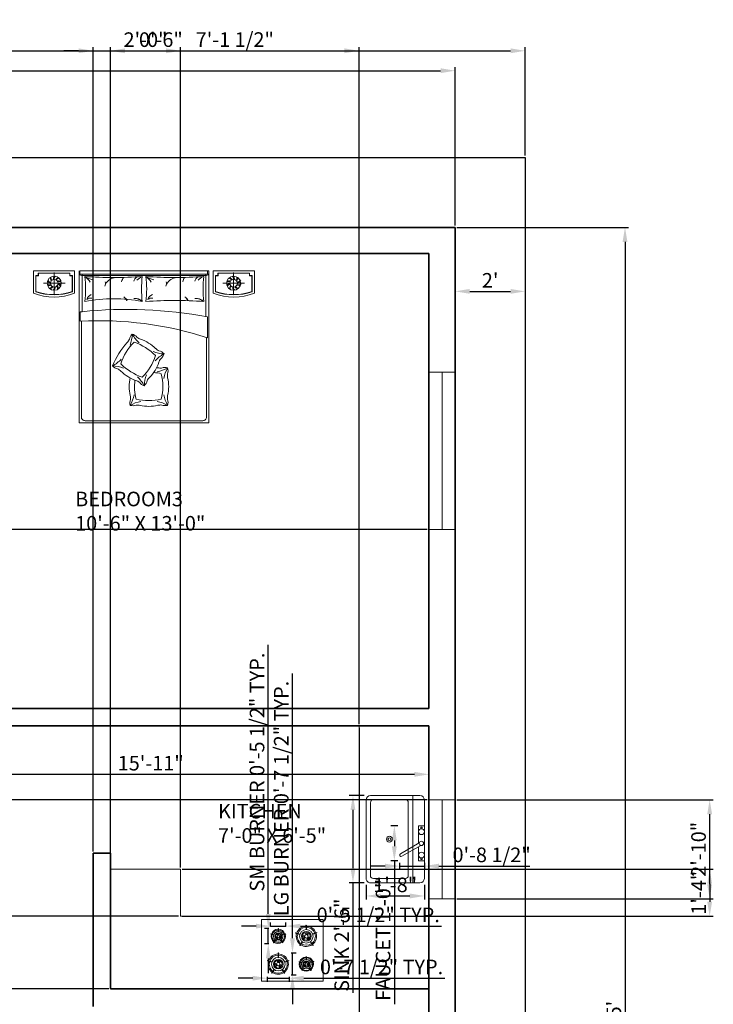
# Model space of a CAD drawing. Units: inches. Extents: x -938 to -211, y -366 to 366.
# Tile 4 of 4: x -450 to -211, y 4 to 341. Entities that reach past the tile are written whole.
import ezdxf

# ---------------------------------------------------------------- set-up
doc = ezdxf.new("R2010")
doc.units = ezdxf.units.IN
doc.header["$PDMODE"] = 35
doc.header["$PDSIZE"] = 5
for name, color, linetype, lineweight in [('A-ANNO-DIMS', 2, 'Continuous', 18), ('A-AREA-IDEN', 7, 'Continuous', 18), ('A-EQPM', 8, 'Continuous', 18), ('A-FLOR-CASE', 32, 'Continuous', 18), ('A-FLOR-FIXT', 9, 'Continuous', 18), ('A-GLAZ', 4, 'Continuous', 18), ('A-WALL', 7, 'Continuous', 35), ('C-PROP', 8, 'Continuous', 25), ('furn', 28, 'Continuous', 13)]:
    doc.layers.add(name, color=color, linetype=linetype, lineweight=lineweight)
doc.styles.get("Standard").update_dxf_attribs({"font": 'arial.ttf'})
doc.dimstyles.new('ISO-25', dxfattribs={"dimtxt": 5, "dimasz": 5, "dimexe": 1.25, "dimexo": 0.625, "dimtad": 1, "dimlunit": 3, "dimtxsty": 'Standard', "dimcen": 2.5, "dimadec": 0, "dimazin": 0, "dimtfac": 1, "dimtmove": 0, "dimatfit": 3, "dimfxl": 1, "dimarcsym": 0})

# ---------------------------------------------------------------- blocks, each defined once
blk = doc.blocks.new('Sink-single - 30 in top')
blk.add_line((-15, -3.999996), (15, -3.999996))
for points in [[(-13.5, 0), (13.5, 0)], [(-15, -18.499996), (-15, -1.5)], [(15, -1.5), (15, -18.499996)], [(-13.5, -17.499996), (-13.5, -6.499996)], [(-12.5, -5.499996), (12.5, -5.499996)], [(13.5, -6.499996), (13.5, -17.499996)], [(13.5, -19.999996), (-13.5, -19.999996)], [(12.5, -18.499996), (-12.5, -18.499996)]]:
    blk.add_lwpolyline(points)
for radius in [1, 0.5]:
    blk.add_circle((0, -11.999996), radius)
for centre, radius, start, end in [((-13.5, -1.5), 1.5, 90, 180), ((13.5, -1.5), 1.5, 0, 90), ((-12.5, -6.499996), 1, 90, 180), ((12.5, -6.499996), 1, 0, 90), ((-13.5, -18.499996), 1.5, 180, 270), ((-12.5, -17.499996), 1, 180, 270), ((12.5, -17.499996), 1, 270, 0), ((13.5, -18.499996), 1.5, 270, 0)]:
    blk.add_arc(centre, radius, start, end)
blk = doc.blocks.new('Faucet - kit sink top')
for p, q in [((-5.5, -0.75), (-5.5, -1.25)), ((-4.94278, -0.75), (-5.5, -0.75)), ((-5.5, -1.25), (-4.94278, -1.25)), ((-0.14775, -1.7441), (3.56698, -8.1782)), ((4.43301, -7.6782), (0.71828, -1.2441)), ((4.94278, -0.75), (5.5, -0.75)), ((5.5, -1.25), (4.94278, -1.25)), ((5.5, -0.75), (5.5, -1.25))]:
    blk.add_line(p, q)
blk.add_lwpolyline([(-0.00587, -2), (-6, -2), (-6, 0), (6, 0), (6, -2), (1.15195, -2)])
for centre, radius in [((-4, -1), 1), ((4, -1), 1), ((0, -1), 0.75)]:
    blk.add_circle(centre, radius)
blk.add_arc((4, -7.9282), 0.5, 210, 30)
blk = doc.blocks.new('*D9')
at = {"layer": 'A-ANNO-DIMS', "color": 0, "lineweight": -2, "transparency": 16777216}
for p, q in [((-500.06, 98.36), (-500.06, 81.14)), ((-309.06, 98.36), (-309.06, 81.14)), ((-495.06, 82.39), (-314.06, 82.39))]:
    blk.add_line(p, q, dxfattribs=at)
at = {"layer": 'A-ANNO-DIMS', "color": 0, "transparency": 16777216}
for points in [[(-495.06, 83.22), (-495.06, 81.55), (-500.06, 82.39)], [(-314.06, 83.22), (-314.06, 81.55), (-309.06, 82.39)]]:
    blk.add_solid(points, dxfattribs=at)
at = {"layer": 'Defpoints', "color": 0, "transparency": 16777216}
for p in [(-500.06, 98.98), (-309.06, 98.98), (-309.06, 82.39)]:
    blk.add_point(p, dxfattribs=at)
at = {"layer": 'A-ANNO-DIMS', "color": 0, "transparency": 16777216, "insert": (-404.56, 85.56), "char_height": 5, "attachment_point": 5}
blk.add_mtext('15\'-11"', dxfattribs=at)
blk = doc.blocks.new('*D19')
at = {"layer": 'A-ANNO-DIMS', "color": 0, "lineweight": -2, "transparency": 16777216}
for p, q in [((-300.06, 253.09), (-300.06, 246.77)), ((-276.06, 253.09), (-276.06, 246.77)), ((-295.06, 248.02), (-281.06, 248.02))]:
    blk.add_line(p, q, dxfattribs=at)
at = {"layer": 'A-ANNO-DIMS', "color": 0, "transparency": 16777216}
for points in [[(-295.06, 248.85), (-295.06, 247.19), (-300.06, 248.02)], [(-281.06, 248.85), (-281.06, 247.19), (-276.06, 248.02)]]:
    blk.add_solid(points, dxfattribs=at)
at = {"layer": 'Defpoints', "color": 0, "transparency": 16777216}
for p in [(-300.06, 253.71), (-276.06, 253.71), (-276.06, 248.02)]:
    blk.add_point(p, dxfattribs=at)
at = {"layer": 'A-ANNO-DIMS', "color": 0, "transparency": 16777216, "insert": (-288.06, 251.16), "char_height": 5, "attachment_point": 5}
blk.add_mtext("2'", dxfattribs=at)
blk = doc.blocks.new('*D22')
at = {"layer": 'A-ANNO-DIMS', "color": 0, "lineweight": -2, "transparency": 16777216}
for p, q in [((-840.06, 270.61), (-840.06, 324.96)), ((-300.06, 270.61), (-300.06, 324.96)), ((-835.06, 323.71), (-305.06, 323.71))]:
    blk.add_line(p, q, dxfattribs=at)
at = {"layer": 'A-ANNO-DIMS', "color": 0, "transparency": 16777216}
for points in [[(-835.06, 324.54), (-835.06, 322.87), (-840.06, 323.71)], [(-305.06, 324.54), (-305.06, 322.87), (-300.06, 323.71)]]:
    blk.add_solid(points, dxfattribs=at)
at = {"layer": 'Defpoints', "color": 0, "transparency": 16777216}
for p in [(-300.06, 323.71), (-840.06, 269.98), (-300.06, 269.98)]:
    blk.add_point(p, dxfattribs=at)
at = {"layer": 'A-ANNO-DIMS', "color": 0, "transparency": 16777216, "insert": (-570.06, 326.87), "char_height": 5, "attachment_point": 5}
blk.add_mtext("45'", dxfattribs=at)
blk = doc.blocks.new('*D23')
at = {"layer": 'A-ANNO-DIMS', "color": 0, "lineweight": -2, "transparency": 16777216}
for p, q in [((-299.44, 269.98), (-240.52, 269.98)), ((-241.77, 264.98), (-241.77, -265.02)), ((-299.44, -270.02), (-240.52, -270.02))]:
    blk.add_line(p, q, dxfattribs=at)
at = {"layer": 'A-ANNO-DIMS', "color": 0, "transparency": 16777216}
for points in [[(-242.61, 264.98), (-240.94, 264.98), (-241.77, 269.98)], [(-242.61, -265.02), (-240.94, -265.02), (-241.77, -270.02)]]:
    blk.add_solid(points, dxfattribs=at)
at = {"layer": 'Defpoints', "color": 0, "transparency": 16777216}
for p in [(-300.06, 269.98), (-300.06, -270.02), (-241.77, -270.02)]:
    blk.add_point(p, dxfattribs=at)
at = {"layer": 'A-ANNO-DIMS', "color": 0, "transparency": 16777216, "insert": (-244.94, -0.02), "char_height": 5, "attachment_point": 5, "rotation": 90}
blk.add_mtext("45'", dxfattribs=at)
blk = doc.blocks.new('BED-DOUBLE-WITH-NIGHTSTANDS')
for p, q in [((-30.77, -7.97), (-30.77, -0.55)), ((-21.46, -1.59), (21.46, -1.59)), ((-21.24, -1.21), (-21.24, -14.04)), ((21.22, -1.21), (21.22, -15.71)), ((30.77, -7.97), (30.77, -0.55)), ((-34.48, -4.26), (-27.06, -4.26)), ((34.48, -4.26), (27.06, -4.26))]:
    blk.add_line(p, q)
for points in [[(-37.91, -7.71), (-37.91, 0), (-23.78, 0), (-23.78, -7.71, -0.181818)], [(-20.26, -10.53, 0.058596), (-20.26, -1.94, 0.036889), (-0.58, -1.94, 0.052163), (-0.58, -10.53, 0.093111)], [(0.7, -10.53, 0.058596), (0.7, -1.94, 0.036648), (20.51, -1.94, 0.052163), (20.51, -10.53, 0.036967)], [(37.91, -7.71), (37.91, 0), (23.78, 0), (23.78, -7.71, 0.181818)], [(-21.84, -14.04), (-21.24, -14.04, -0.072944), (21.82, -15.84), (21.82, -22.97, 0.092568), (-21.84, -17.31)]]:
    blk.add_lwpolyline(points, format="xyb", close=True)
for points in [[(-36.29, -0.77), (-36.29, -1.62), (-37.14, -1.62)], [(-36.22, -0.77), (-36.22, -1.7), (-37.14, -1.7)], [(-36.29, -0.77), (-25.39, -0.77)], [(-36.29, -0.85), (-25.39, -0.85)], [(-25.47, -0.77), (-25.47, -1.7), (-24.55, -1.7)], [(-25.39, -0.77), (-25.39, -1.62), (-24.55, -1.62)], [(-22.23, 0), (-22.23, -52.18), (22.23, -52.18), (22.23, 0)], [(21.82, 0), (21.82, -1.21), (-21.98, -1.21), (-21.98, 0), (22.23, 0)], [(25.39, -0.77), (25.39, -1.62), (24.55, -1.62)], [(25.47, -0.77), (25.47, -1.7), (24.55, -1.7)], [(36.29, -0.77), (25.39, -0.77)], [(36.29, -0.85), (25.39, -0.85)], [(36.22, -0.77), (36.22, -1.7), (37.14, -1.7)], [(36.29, -0.77), (36.29, -1.62), (37.14, -1.62)]]:
    blk.add_lwpolyline(points)
for points in [[(-24.55, -1.62), (-24.55, -7.18, -0.167087), (-37.14, -7.18), (-37.14, -1.62)], [(-24.62, -1.62), (-24.62, -7.12, -0.165559), (-37.06, -7.12), (-37.06, -1.62)], [(24.55, -1.62), (24.55, -7.17, 0.167087), (37.14, -7.17), (37.14, -1.62)], [(24.62, -1.62), (24.62, -7.12, 0.165559), (37.06, -7.12), (37.06, -1.62)], [(-21.46, -17.29), (-21.46, -50.12, 0.414214), (-20.18, -51.41), (20.18, -51.41, 0.414214), (21.46, -50.12), (21.46, -22.84)], [(-4.77, -25.48, 0.091296), (-3.99, -21.71, 0.091296), (-1.62, -24.74, 0.091296)], [(-7.96, -31.91, 0.111006), (-0.61, -36.48, 0.119549), (4.01, -29.05, 0.107813), (-3.31, -24.46)], [(-3.34, -24.47, 0.121865), (-7.96, -31.91, 0.121865)], [(-7.02, -33.41, 0.091296), (-10.79, -32.62, 0.091296), (-7.75, -30.26, 0.091296)], [(0.12, -39.42, 0.159461), (1.12, -37.65, -0.076283), (1.91, -36.55, 0.115075), (5.13, -31.37, -0.076283), (5.77, -30.18, 0.159461), (6.92, -28.51)], [(3.15, -27.72, 0.091296), (6.92, -28.51, 0.091296), (3.88, -30.87, 0.091296)], [(4.54, -34.62, 0.091296), (8.15, -33.3, 0.091296), (6.83, -36.91, 0.091296)], [(8.15, -46.15, 0.159461), (8.07, -44.13, -0.076283), (8.15, -42.78, 0.115075), (8.15, -36.68, -0.076283), (8.07, -35.33, 0.159461), (8.15, -33.3)], [(-2.67, -44.06, 0.111006), (5.98, -44.05, 0.119549), (5.98, -35.3, 0.033212), (3.32, -34.89)], [(0.9, -35.65, 0.091296), (0.12, -39.42, 0.091296), (-2.25, -36.39)], [(-1.08, -44.84, 0.091296), (-4.7, -46.15, 0.091296), (-3.37, -42.55, 0.091296)], [(6.83, -42.55, 0.091296), (8.15, -46.15, 0.091296), (4.54, -44.84)]]:
    blk.add_lwpolyline(points, format="xyb")
for centre, radius in [((-30.77, -4.26), 2.42), ((-30.77, -4.26), 1.31), ((30.77, -4.26), 2.42), ((30.77, -4.26), 1.31)]:
    blk.add_circle(centre, radius)
for centre, radius, start, end in [((-31.77, -2.78), 1.19, 196.3002, 256.538), ((-30.56, -2.45), 1.56, 172.17, 218.4897), ((-30.71, -2.48), 1.19, 160.3002, 220.538), ((-29.53, -2.92), 1.56, 136.17, 182.4897), ((-29.67, -2.86), 1.19, 124.3002, 184.538), ((-28.98, -3.9), 1.56, 100.17, 146.4897), ((-29.06, -3.77), 1.19, 88.3002, 148.538), ((-21.46, -0.82), 0.771, 180, 270), ((-15.69, 5.24), 8.51, 237.5379, 257.5233), ((-26.7, -9.98), 10.3, 36.4935, 51.2792), ((-9.16, -7.04), 4.76, 96.6849, 148.3182), ((-4.35, -4.33), 3.34, 141.8174, 169.8987), ((-0.12, -4.8), 3.6, 130.5354, 160.3558), ((2.12, -7.83), 6.48, 114.6457, 134.1585), ((-5.74, -9.98), 10.3, 36.4935, 51.2792), ((5.27, 5.24), 8.51, 237.5379, 257.5233), ((11.8, -7.04), 4.76, 96.6849, 148.3182), ((16.61, -4.33), 3.34, 141.8174, 169.8987), ((20.84, -4.8), 3.6, 130.5354, 160.3558), ((23.08, -7.83), 6.48, 114.6457, 134.1585), ((21.46, -0.82), 0.771, 270, 0), ((29.06, -3.77), 1.19, 31.462, 91.6998), ((28.98, -3.9), 1.56, 33.5103, 79.83), ((29.67, -2.86), 1.19, 355.462, 55.6998), ((29.53, -2.92), 1.56, 357.5103, 43.83), ((30.71, -2.48), 1.19, 319.462, 19.6998), ((30.73, -2.38), 1.56, 321.5103, 7.83), ((31.94, -2.72), 1.19, 283.462, 343.6998), ((31.84, -2.6), 1.56, 285.5103, 331.83), ((-32.44, -3.65), 1.19, 232.3002, 292.538), ((-32.43, -3.5), 1.56, 244.17, 290.4897), ((-31.66, -2.67), 1.56, 208.17, 254.4897), ((-32.48, -4.75), 1.19, 268.3002, 328.538), ((-32.56, -4.62), 1.56, 280.17, 326.4897), ((-31.87, -5.66), 1.19, 304.3002, 4.538), ((-32.01, -5.6), 1.56, 316.17, 2.4897), ((-30.83, -6.04), 1.19, 340.3002, 40.538), ((-30.99, -6.07), 1.56, 352.17, 38.4897), ((-29.11, -5.02), 1.56, 64.17, 110.4897), ((-29.1, -4.87), 1.19, 52.3002, 112.538), ((-29.78, -5.74), 1.19, 16.3002, 76.538), ((-29.88, -5.85), 1.56, 28.17, 74.4897), ((-15.35, -4.38), 2.13, 335.8927, 16.1192), ((5.61, -4.38), 2.13, 335.8927, 16.1192), ((29.1, -4.87), 1.19, 67.462, 127.6998), ((29.11, -5.03), 1.56, 69.5103, 115.83), ((29.88, -5.85), 1.56, 105.5103, 151.83), ((29.78, -5.74), 1.19, 103.462, 163.6998), ((30.99, -6.07), 1.56, 141.5103, 187.83), ((30.83, -6.04), 1.19, 139.462, 199.6998), ((32.01, -5.6), 1.56, 177.5103, 223.83), ((31.87, -5.66), 1.19, 175.462, 235.6998), ((32.56, -4.62), 1.56, 213.5103, 259.83), ((32.48, -4.75), 1.19, 211.462, 271.6998), ((32.61, -3.43), 1.56, 249.5103, 295.83), ((32.62, -3.58), 1.19, 247.462, 307.6998), ((-16.88, -10.73), 2.86, 114.2916, 160.9896), ((-18.36, -11.33), 1.95, 76.4823, 128.5563), ((-14.47, -16.51), 10.73, 36.2085, 45.0849), ((-6.53, -10.17), 0.72, 353.7543, 77.2187), ((-3.09, -12.99), 3.51, 44.406, 96.8342), ((-2.43, -11.76), 2.23, 33.6349, 90.8456), ((4.08, -10.73), 2.86, 114.2916, 160.9896), ((2.6, -11.33), 1.95, 76.4823, 128.5563), ((6.49, -16.51), 10.73, 36.2085, 45.0849), ((14.43, -10.17), 0.72, 353.7543, 77.2187), ((17.87, -12.99), 3.51, 44.406, 96.8342), ((18.53, -11.76), 2.23, 33.6349, 90.8456), ((-8.96, -21.45), 4.46, 315.5854, 333.0343), ((-1.79, -24.12), 3.26, 132.4658, 168.7065), ((-4.85, -24.74), 3.14, 37.2937, 74.0973), ((0.32, -19.25), 4.46, 233.2983, 250.7472), ((-5.44, -36.19), 13.43, 45.1307, 71.3884), ((15.27, -43.27), 28.15, 138.3818, 157.7644), ((7.15, -23.48), 4.46, 225.7718, 243.2208), ((4.59, -30.42), 3.01, 39.4726, 79.6505), ((-8.39, -30.41), 3.26, 222.6522, 258.8929), ((-11.03, -37.59), 4.46, 45.7718, 63.2208), ((1.73, -46.36), 13.43, 77.0576, 78.7033), ((5.69, -28.91), 4.46, 257.6988, 275.1477), ((7.19, -36.15), 3.01, 71.3996, 111.5774), ((1.56, -24.88), 13.43, 225.1307, 251.3884), ((8.38, -39.73), 13.43, 166.8711, 193.1289), ((15.01, -39.64), 18.22, 173.1956, 194.0284), ((-4.2, -41.82), 4.46, 53.2983, 70.7472), ((1.37, -35.91), 3.73, 218.7754, 250.3571), ((-9.05, -43.74), 4.46, 355.0387, 12.4877), ((-1.56, -45.28), 3.26, 159.3666, 195.6073), ((-3.83, -43.01), 3.26, 254.5791, 290.8198), ((-2.27, -50.5), 4.46, 77.6988, 95.1477), ((1.69, -33.06), 13.43, 257.0576, 283.3153), ((5.76, -50.48), 4.46, 85.2252, 102.6741), ((7.36, -42.51), 3.73, 250.7023, 282.284)]:
    blk.add_arc(centre, radius, start, end)
blk = doc.blocks.new('WINDOW-54IN')
blk.add_line((54, 0), (0, 0))
blk.add_lwpolyline([(54, 4.5), (54, -4.5), (0, -4.5), (0, 4.5)], close=True)
blk = doc.blocks.new('COOKTOP-BURNER-LARGE')
for p, q in [((-0.06, 2.38), (-0.06, 3.81)), ((0.06, 2.38), (0.06, 3.81)), ((-2.28, 0.68), (-3.64, 1.12)), ((-2.24, 0.79), (-3.6, 1.23)), ((2.24, 0.79), (3.6, 1.23)), ((2.28, 0.68), (3.64, 1.12)), ((-1.44, -1.89), (-2.28, -3.04)), ((-1.35, -1.96), (-2.19, -3.11)), ((1.35, -1.96), (2.19, -3.11)), ((1.44, -1.89), (2.28, -3.04))]:
    blk.add_line(p, q)
for radius in [2.32, 1.66, 1.35, 0.58]:
    blk.add_circle((0, 0), radius)
for centre, radius, start, end in [((0, 0), 3.48, 90.9557, 161.0457), ((0, 3.81), 0.058, 0.0007, 180.0007), ((0, 0), 3.48, 18.9557, 89.0457), ((-3.62, 1.18), 0.058, 72.0007, 252.0007), ((0, 0), 3.48, 162.9557, 233.0457), ((0, 0), 3.09, 163.075, 232.9263), ((0, 0), 3.09, 91.075, 160.9263), ((-2.26, 0.73), 0.058, 252.0007, 72.0007), ((-0.97, 0), 0.193, 0.0007, 180.0007), ((-0.06, 0.96), 0.193, 93.5265, 273.5265), ((0, 0), 1.16, 60.0007, 93.5265), ((0, 2.38), 0.058, 180.0007, 0.0007), ((0, 0), 0.773, 60.0007, 93.5265), ((0, 0), 3.09, 19.075, 88.9263), ((0.48, 0.84), 0.193, 240.0007, 60.0007), ((0, 0), 3.09, 307.075, 16.9263), ((0, 0), 3.48, 306.9557, 17.0457), ((2.26, 0.73), 0.058, 108.0007, 288.0007), ((3.62, 1.18), 0.058, 288.0007, 108.0007), ((-2.24, -3.08), 0.058, 144.0007, 324.0007), ((0, 0), 3.48, 234.9557, 305.0457), ((0, 0), 3.09, 235.075, 304.9263), ((-1.4, -1.92), 0.058, 324.0007, 144.0007), ((0, 0), 1.16, 180.0007, 213.5265), ((-0.81, -0.53), 0.193, 213.5265, 33.5265), ((0, 0), 0.773, 180.0007, 213.5265), ((0.48, -0.84), 0.193, 120.0007, 300.0007), ((0, 0), 0.773, 300.0007, 333.5265), ((0, 0), 1.16, 300.0007, 333.5265), ((0.87, -0.43), 0.193, 333.5265, 153.5265), ((1.4, -1.92), 0.058, 36.0007, 216.0007), ((2.24, -3.08), 0.058, 216.0007, 36.0007)]:
    blk.add_arc(centre, radius, start, end)
blk = doc.blocks.new('COOKTOP-BURNER-SMALL')
for p, q in [((-1.6, 0.48), (-2.55, 0.78)), ((-1.57, 0.55), (-2.52, 0.86)), ((-0.04, 1.66), (-0.04, 2.66)), ((0.04, 1.66), (0.04, 2.66)), ((1.57, 0.55), (2.52, 0.86)), ((1.6, 0.48), (2.55, 0.78)), ((-1.01, -1.32), (-1.6, -2.13)), ((-0.95, -1.37), (-1.53, -2.18)), ((0.95, -1.37), (1.53, -2.18)), ((1.01, -1.32), (1.6, -2.13))]:
    blk.add_line(p, q)
for radius in [1.62, 1.16, 0.947, 0.406]:
    blk.add_circle((0, 0), radius)
for centre, radius, start, end in [((-2.53, 0.82), 0.0406, 72.0007, 252.0007), ((0, 0), 2.44, 162.9557, 233.0457), ((0, 0), 2.44, 90.9557, 161.0457), ((0, 0), 2.16, 163.075, 232.9263), ((0, 0), 2.16, 91.075, 160.9263), ((-1.58, 0.51), 0.0406, 252.0007, 72.0007), ((-0.34, 0.59), 0.135, 120.0007, 300.0007), ((0, 0), 0.812, 86.4748, 120.0007), ((0, 0), 0.541, 86.4748, 120.0007), ((0, 2.66), 0.0406, 0.0007, 180.0007), ((0, 1.66), 0.0406, 180.0007, 0.0007), ((0.04, 0.68), 0.135, 266.4748, 86.4748), ((0, 0), 2.44, 18.9557, 89.0457), ((0, 0), 2.16, 19.075, 88.9263), ((0, 0), 0.541, 326.4748, 0.0007), ((0.68, 0), 0.135, 0.0007, 180.0007), ((0, 0), 0.812, 326.4748, 0.0007), ((0, 0), 2.16, 307.075, 16.9263), ((0, 0), 2.44, 306.9557, 17.0457), ((1.58, 0.51), 0.0406, 108.0007, 288.0007), ((2.53, 0.82), 0.0406, 288.0007, 108.0007), ((-1.57, -2.16), 0.0406, 144.0007, 324.0007), ((-0.09, 0), 2.44, 234.9557, 305.0457), ((0, 0), 2.16, 235.075, 304.9263), ((-0.98, -1.35), 0.0406, 324.0007, 144.0007), ((-0.61, -0.3), 0.135, 26.4748, 206.4748), ((0, 0), 0.812, 206.4748, 240.0007), ((0, 0), 0.541, 206.4748, 240.0007), ((-0.34, -0.59), 0.135, 240.0007, 60.0007), ((0.56, -0.37), 0.135, 146.4748, 326.4748), ((0.98, -1.35), 0.0406, 36.0007, 216.0007), ((1.57, -2.16), 0.0406, 216.0007, 36.0007)]:
    blk.add_arc(centre, radius, start, end)
blk = doc.blocks.new('*D35')
at = {"layer": 'A-ANNO-DIMS', "color": 0, "lineweight": -2, "transparency": 16777216}
for p, q in [((-355.9, 26.16), (-355.9, 117.01)), ((-356.4, 21.16), (-354.65, 21.16)), ((-355.9, 13.6), (-355.9, 21.16)), ((-356.4, 13.6), (-354.65, 13.6)), ((-355.9, 8.6), (-355.9, 3.6))]:
    blk.add_line(p, q, dxfattribs=at)
at = {"layer": 'A-ANNO-DIMS', "color": 0, "transparency": 16777216}
for points in [[(-356.73, 26.16), (-355.06, 26.16), (-355.9, 21.16)], [(-356.73, 8.6), (-355.06, 8.6), (-355.9, 13.6)]]:
    blk.add_solid(points, dxfattribs=at)
at = {"layer": 'Defpoints', "color": 0, "transparency": 16777216}
for p in [(-357.03, 21.16), (-355.9, 21.16), (-357.03, 13.6)]:
    blk.add_point(p, dxfattribs=at)
at = {"layer": 'A-ANNO-DIMS', "color": 0, "transparency": 16777216, "insert": (-359.11, 74.08), "char_height": 5, "attachment_point": 5, "rotation": 90}
blk.add_mtext('LG BURNER 0\'-7 1/2" TYP.', dxfattribs=at)
blk = doc.blocks.new('*D36')
at = {"layer": 'A-ANNO-DIMS', "color": 0, "lineweight": -2, "transparency": 16777216}
for p, q in [((-369.54, 12.47), (-374.54, 12.47)), ((-364.54, 12.98), (-364.54, 11.22)), ((-364.54, 12.47), (-357.03, 12.47)), ((-357.03, 12.98), (-357.03, 11.22)), ((-352.03, 12.47), (-303.65, 12.47))]:
    blk.add_line(p, q, dxfattribs=at)
at = {"layer": 'A-ANNO-DIMS', "color": 0, "transparency": 16777216}
for points in [[(-369.54, 13.3), (-369.54, 11.64), (-364.54, 12.47)], [(-352.03, 13.3), (-352.03, 11.64), (-357.03, 12.47)]]:
    blk.add_solid(points, dxfattribs=at)
at = {"layer": 'Defpoints', "color": 0, "transparency": 16777216}
for p in [(-364.54, 13.6), (-357.03, 13.6), (-357.03, 12.47)]:
    blk.add_point(p, dxfattribs=at)
at = {"layer": 'A-ANNO-DIMS', "color": 0, "transparency": 16777216, "insert": (-325.34, 15.68), "char_height": 5, "attachment_point": 5}
blk.add_mtext('0\'-7 1/2" TYP.', dxfattribs=at)
blk = doc.blocks.new('*D37')
at = {"layer": 'A-ANNO-DIMS', "color": 0, "lineweight": -2, "transparency": 16777216}
for p, q in [((-364.21, 34.54), (-364.21, 126.75)), ((-364.04, 29.54), (-365.46, 29.54)), ((-364.21, 24.25), (-364.21, 29.54)), ((-364.04, 24.25), (-365.46, 24.25)), ((-364.21, 19.25), (-364.21, 14.25))]:
    blk.add_line(p, q, dxfattribs=at)
at = {"layer": 'A-ANNO-DIMS', "color": 0, "transparency": 16777216}
for points in [[(-365.04, 34.54), (-363.37, 34.54), (-364.21, 29.54)], [(-365.04, 19.25), (-363.37, 19.25), (-364.21, 24.25)]]:
    blk.add_solid(points, dxfattribs=at)
at = {"layer": 'Defpoints', "color": 0, "transparency": 16777216}
for p in [(-364.21, 29.54), (-363.41, 29.54), (-363.41, 24.25)]:
    blk.add_point(p, dxfattribs=at)
at = {"layer": 'A-ANNO-DIMS', "color": 0, "transparency": 16777216, "insert": (-367.42, 83.14), "char_height": 5, "attachment_point": 5, "rotation": 90}
blk.add_mtext('SM BURNER 0\'-5 1/2" TYP.', dxfattribs=at)
blk = doc.blocks.new('*D38')
at = {"layer": 'A-ANNO-DIMS', "color": 0, "lineweight": -2, "transparency": 16777216}
for p, q in [((-363.41, 30.16), (-363.41, 31.58)), ((-358.16, 30.16), (-358.16, 31.58)), ((-368.41, 30.33), (-373.41, 30.33)), ((-363.41, 30.33), (-358.16, 30.33)), ((-353.16, 30.33), (-304.78, 30.33))]:
    blk.add_line(p, q, dxfattribs=at)
at = {"layer": 'A-ANNO-DIMS', "color": 0, "transparency": 16777216}
for points in [[(-368.41, 31.16), (-368.41, 29.5), (-363.41, 30.33)], [(-353.16, 31.16), (-353.16, 29.5), (-358.16, 30.33)]]:
    blk.add_solid(points, dxfattribs=at)
at = {"layer": 'Defpoints', "color": 0, "transparency": 16777216}
for p in [(-363.41, 29.54), (-358.16, 30.33), (-358.16, 29.54)]:
    blk.add_point(p, dxfattribs=at)
at = {"layer": 'A-ANNO-DIMS', "color": 0, "transparency": 16777216, "insert": (-326.47, 33.54), "char_height": 5, "attachment_point": 5}
blk.add_mtext('0\'-5 1/2" TYP.', dxfattribs=at)
blk = doc.blocks.new('*D39')
at = {"layer": 'A-ANNO-DIMS', "color": 0, "lineweight": -2, "transparency": 16777216}
for p, q in [((-331.27, 75.17), (-336.39, 75.17)), ((-335.14, 70.17), (-335.14, 50.17)), ((-331.27, 45.17), (-336.39, 45.17)), ((-335.14, 45.17), (-335.14, 7.4))]:
    blk.add_line(p, q, dxfattribs=at)
at = {"layer": 'A-ANNO-DIMS', "color": 0, "transparency": 16777216}
for points in [[(-335.98, 70.17), (-334.31, 70.17), (-335.14, 75.17)], [(-335.98, 50.17), (-334.31, 50.17), (-335.14, 45.17)]]:
    blk.add_solid(points, dxfattribs=at)
at = {"layer": 'Defpoints', "color": 0, "transparency": 16777216}
for p in [(-330.64, 75.17), (-335.14, 45.17), (-330.64, 45.17)]:
    blk.add_point(p, dxfattribs=at)
at = {"layer": 'A-ANNO-DIMS', "color": 0, "transparency": 16777216, "insert": (-338.36, 23.78), "char_height": 5, "attachment_point": 5, "rotation": 90}
blk.add_mtext('SINK 2\'-6"', dxfattribs=at)
blk = doc.blocks.new('*D40')
at = {"layer": 'A-ANNO-DIMS', "color": 0, "lineweight": -2, "transparency": 16777216}
for p, q in [((-330.64, 44.54), (-330.64, 39.42)), ((-310.64, 44.54), (-310.64, 39.42)), ((-325.64, 40.67), (-315.64, 40.67))]:
    blk.add_line(p, q, dxfattribs=at)
at = {"layer": 'A-ANNO-DIMS', "color": 0, "transparency": 16777216}
for points in [[(-325.64, 41.5), (-325.64, 39.83), (-330.64, 40.67)], [(-315.64, 41.5), (-315.64, 39.83), (-310.64, 40.67)]]:
    blk.add_solid(points, dxfattribs=at)
at = {"layer": 'Defpoints', "color": 0, "transparency": 16777216}
for p in [(-330.64, 45.17), (-310.64, 45.17), (-310.64, 40.67)]:
    blk.add_point(p, dxfattribs=at)
at = {"layer": 'A-ANNO-DIMS', "color": 0, "transparency": 16777216, "insert": (-320.64, 43.84), "char_height": 5, "attachment_point": 5}
blk.add_mtext('1\'-8"', dxfattribs=at)
blk = doc.blocks.new('*D41')
at = {"layer": 'A-ANNO-DIMS', "color": 0, "lineweight": -2, "transparency": 16777216}
for p, q in [((-319.77, 64.71), (-322.19, 64.71)), ((-320.94, 59.71), (-320.94, 57.71)), ((-319.77, 52.71), (-322.19, 52.71)), ((-320.94, 52.71), (-320.94, 3.57))]:
    blk.add_line(p, q, dxfattribs=at)
at = {"layer": 'A-ANNO-DIMS', "color": 0, "transparency": 16777216}
for points in [[(-321.78, 59.71), (-320.11, 59.71), (-320.94, 64.71)], [(-321.78, 57.71), (-320.11, 57.71), (-320.94, 52.71)]]:
    blk.add_solid(points, dxfattribs=at)
at = {"layer": 'Defpoints', "color": 0, "transparency": 16777216}
for p in [(-319.14, 64.71), (-320.94, 52.71), (-319.14, 52.71)]:
    blk.add_point(p, dxfattribs=at)
at = {"layer": 'A-ANNO-DIMS', "color": 0, "transparency": 16777216, "insert": (-324.15, 25.64), "char_height": 5, "attachment_point": 5, "rotation": 90}
blk.add_mtext('FAUCET 1\'-0"', dxfattribs=at)
blk = doc.blocks.new('*D42')
at = {"layer": 'A-ANNO-DIMS', "color": 0, "lineweight": -2, "transparency": 16777216}
for p, q in [((-324.14, 50.91), (-329.14, 50.91)), ((-319.14, 52.09), (-319.14, 49.66)), ((-319.14, 50.91), (-310.64, 50.91)), ((-310.64, 52.09), (-310.64, 49.66)), ((-305.64, 50.91), (-274.45, 50.91))]:
    blk.add_line(p, q, dxfattribs=at)
at = {"layer": 'A-ANNO-DIMS', "color": 0, "transparency": 16777216}
for points in [[(-324.14, 51.74), (-324.14, 50.08), (-319.14, 50.91)], [(-305.64, 51.74), (-305.64, 50.08), (-310.64, 50.91)]]:
    blk.add_solid(points, dxfattribs=at)
at = {"layer": 'Defpoints', "color": 0, "transparency": 16777216}
for p in [(-319.14, 52.71), (-310.64, 52.71), (-310.64, 50.91)]:
    blk.add_point(p, dxfattribs=at)
at = {"layer": 'A-ANNO-DIMS', "color": 0, "transparency": 16777216, "insert": (-287.55, 54.12), "char_height": 5, "attachment_point": 5}
blk.add_mtext('0\'-8 1/2"', dxfattribs=at)
blk = doc.blocks.new('*D43')
at = {"layer": 'A-ANNO-DIMS', "color": 0, "lineweight": -2, "transparency": 16777216}
for p, q in [((-876.06, 294.61), (-876.06, 331.78)), ((-276.06, 294.61), (-276.06, 331.78)), ((-871.06, 330.53), (-281.06, 330.53))]:
    blk.add_line(p, q, dxfattribs=at)
at = {"layer": 'A-ANNO-DIMS', "color": 0, "transparency": 16777216}
for points in [[(-871.06, 331.37), (-871.06, 329.7), (-876.06, 330.53)], [(-281.06, 331.37), (-281.06, 329.7), (-276.06, 330.53)]]:
    blk.add_solid(points, dxfattribs=at)
at = {"layer": 'Defpoints', "color": 0, "transparency": 16777216}
for p in [(-276.06, 330.53), (-876.06, 293.98), (-276.06, 293.98)]:
    blk.add_point(p, dxfattribs=at)
at = {"layer": 'A-ANNO-DIMS', "color": 0, "transparency": 16777216, "insert": (-576.06, 333.71), "char_height": 5, "attachment_point": 5}
blk.add_mtext('50\'-0"', dxfattribs=at)
blk = doc.blocks.new('*D50')
at = {"layer": 'A-ANNO-DIMS', "color": 0, "lineweight": -2, "transparency": 16777216}
for p, q in [((-333.06, 98.36), (-333.06, -363.01)), ((-309.06, 98.36), (-309.06, -363.01)), ((-328.06, -361.76), (-314.06, -361.76))]:
    blk.add_line(p, q, dxfattribs=at)
at = {"layer": 'A-ANNO-DIMS', "color": 0, "transparency": 16777216}
for points in [[(-328.06, -360.93), (-328.06, -362.6), (-333.06, -361.76)], [(-314.06, -360.93), (-314.06, -362.6), (-309.06, -361.76)]]:
    blk.add_solid(points, dxfattribs=at)
at = {"layer": 'Defpoints', "color": 0, "transparency": 16777216}
for p in [(-333.06, 98.98), (-309.06, 98.98), (-309.06, -361.76)]:
    blk.add_point(p, dxfattribs=at)
at = {"layer": 'A-ANNO-DIMS', "color": 0, "transparency": 16777216, "insert": (-321.06, -358.59), "char_height": 5, "attachment_point": 5}
blk.add_mtext('2\'-0"', dxfattribs=at)
blk = doc.blocks.new('*D56')
at = {"layer": 'A-ANNO-DIMS', "color": 0, "lineweight": -2, "transparency": 16777216}
for p, q in [((-309.69, 166.31), (-928.86, 166.31)), ((-927.61, 109.98), (-927.61, 161.31)), ((-309.69, 104.98), (-928.86, 104.98))]:
    blk.add_line(p, q, dxfattribs=at)
at = {"layer": 'A-ANNO-DIMS', "color": 0, "transparency": 16777216}
for points in [[(-928.45, 161.31), (-926.78, 161.31), (-927.61, 166.31)], [(-928.45, 109.98), (-926.78, 109.98), (-927.61, 104.98)]]:
    blk.add_solid(points, dxfattribs=at)
at = {"layer": 'Defpoints', "color": 0, "transparency": 16777216}
for p in [(-927.61, 166.31), (-309.06, 166.31), (-309.06, 104.98)]:
    blk.add_point(p, dxfattribs=at)
at = {"layer": 'A-ANNO-DIMS', "color": 0, "transparency": 16777216, "insert": (-930.82, 135.65), "char_height": 5, "attachment_point": 5, "rotation": 90}
blk.add_mtext('5\'-1 1/2"', dxfattribs=at)
blk = doc.blocks.new('*D59')
at = {"layer": 'A-ANNO-DIMS', "color": 0, "lineweight": -2, "transparency": 16777216}
for p, q in [((-299.44, 73.67), (-211.46, 73.67)), ((-212.71, 44.67), (-212.71, 68.67)), ((-299.44, 39.67), (-211.46, 39.67))]:
    blk.add_line(p, q, dxfattribs=at)
at = {"layer": 'A-ANNO-DIMS', "color": 0, "transparency": 16777216}
for points in [[(-213.55, 68.67), (-211.88, 68.67), (-212.71, 73.67)], [(-213.55, 44.67), (-211.88, 44.67), (-212.71, 39.67)]]:
    blk.add_solid(points, dxfattribs=at)
at = {"layer": 'Defpoints', "color": 0, "transparency": 16777216}
for p in [(-300.06, 73.67), (-212.71, 73.67), (-300.06, 39.67)]:
    blk.add_point(p, dxfattribs=at)
at = {"layer": 'A-ANNO-DIMS', "color": 0, "transparency": 16777216, "insert": (-215.89, 56.67), "char_height": 5, "attachment_point": 5, "rotation": 90}
blk.add_mtext('2\'-10"', dxfattribs=at)
blk = doc.blocks.new('*D60')
at = {"layer": 'A-ANNO-DIMS', "color": 0, "lineweight": -2, "transparency": 16777216}
for p, q in [((-394.97, 33.71), (-928.86, 33.71)), ((-927.61, 28.71), (-927.61, 13.79)), ((-418.97, 8.79), (-928.86, 8.79))]:
    blk.add_line(p, q, dxfattribs=at)
at = {"layer": 'A-ANNO-DIMS', "color": 0, "transparency": 16777216}
for points in [[(-928.45, 28.71), (-926.78, 28.71), (-927.61, 33.71)], [(-928.45, 13.79), (-926.78, 13.79), (-927.61, 8.79)]]:
    blk.add_solid(points, dxfattribs=at)
at = {"layer": 'Defpoints', "color": 0, "transparency": 16777216}
for p in [(-394.34, 33.71), (-927.61, 8.79), (-418.34, 8.79)]:
    blk.add_point(p, dxfattribs=at)
at = {"layer": 'A-ANNO-DIMS', "color": 0, "transparency": 16777216, "insert": (-930.75, 21.25), "char_height": 5, "attachment_point": 5, "rotation": 90}
blk.add_mtext('2\'-1"', dxfattribs=at)
blk = doc.blocks.new('*D61')
at = {"layer": 'A-ANNO-DIMS', "color": 0, "lineweight": -2, "transparency": 16777216}
for p, q in [((-424.34, 55.97), (-424.34, 331.78)), ((-418.34, 55.97), (-418.34, 331.78)), ((-429.34, 330.53), (-434.34, 330.53)), ((-424.34, 330.53), (-418.34, 330.53)), ((-413.34, 330.53), (-393.8, 330.53))]:
    blk.add_line(p, q, dxfattribs=at)
at = {"layer": 'A-ANNO-DIMS', "color": 0, "transparency": 16777216}
for points in [[(-429.34, 331.37), (-429.34, 329.7), (-424.34, 330.53)], [(-413.34, 331.37), (-413.34, 329.7), (-418.34, 330.53)]]:
    blk.add_solid(points, dxfattribs=at)
at = {"layer": 'Defpoints', "color": 0, "transparency": 16777216}
for p in [(-418.34, 330.53), (-424.34, 55.34), (-418.34, 55.34)]:
    blk.add_point(p, dxfattribs=at)
at = {"layer": 'A-ANNO-DIMS', "color": 0, "transparency": 16777216, "insert": (-401.07, 333.71), "char_height": 5, "attachment_point": 5}
blk.add_mtext('0\'-6"', dxfattribs=at)
blk = doc.blocks.new('*D64')
at = {"layer": 'A-ANNO-DIMS', "color": 0, "lineweight": -2, "transparency": 16777216}
for p, q in [((-418.34, 50.48), (-418.34, 331.78)), ((-394.34, 50.48), (-394.34, 331.78)), ((-413.34, 330.53), (-399.34, 330.53))]:
    blk.add_line(p, q, dxfattribs=at)
at = {"layer": 'A-ANNO-DIMS', "color": 0, "transparency": 16777216}
for points in [[(-413.34, 331.37), (-413.34, 329.7), (-418.34, 330.53)], [(-399.34, 331.37), (-399.34, 329.7), (-394.34, 330.53)]]:
    blk.add_solid(points, dxfattribs=at)
at = {"layer": 'Defpoints', "color": 0, "transparency": 16777216}
for p in [(-394.34, 330.53), (-418.34, 49.85), (-394.34, 49.85)]:
    blk.add_point(p, dxfattribs=at)
at = {"layer": 'A-ANNO-DIMS', "color": 0, "transparency": 16777216, "insert": (-406.34, 333.71), "char_height": 5, "attachment_point": 5}
blk.add_mtext('2\'-0"', dxfattribs=at)
blk = doc.blocks.new('*D65')
at = {"layer": 'A-ANNO-DIMS', "color": 0, "lineweight": -2, "transparency": 16777216}
for p, q in [((-393.72, 49.85), (-211.46, 49.85)), ((-212.71, 44.85), (-212.71, 38.71)), ((-393.72, 33.71), (-211.46, 33.71))]:
    blk.add_line(p, q, dxfattribs=at)
at = {"layer": 'A-ANNO-DIMS', "color": 0, "transparency": 16777216}
for points in [[(-213.55, 44.85), (-211.88, 44.85), (-212.71, 49.85)], [(-213.55, 38.71), (-211.88, 38.71), (-212.71, 33.71)]]:
    blk.add_solid(points, dxfattribs=at)
at = {"layer": 'Defpoints', "color": 0, "transparency": 16777216}
for p in [(-394.34, 49.85), (-394.34, 33.71), (-212.71, 33.71)]:
    blk.add_point(p, dxfattribs=at)
at = {"layer": 'A-ANNO-DIMS', "color": 0, "transparency": 16777216, "insert": (-215.85, 41.78), "char_height": 5, "attachment_point": 5, "rotation": 90}
blk.add_mtext('1\'-4"', dxfattribs=at)
blk = doc.blocks.new('*D66')
at = {"layer": 'A-ANNO-DIMS', "color": 0, "lineweight": -2, "transparency": 16777216}
for p, q in [((-309.69, 98.98), (-928.86, 98.98)), ((-927.61, 93.98), (-927.61, 78.67)), ((-309.69, 73.67), (-928.86, 73.67)), ((-927.61, 73.67), (-927.61, 42.39))]:
    blk.add_line(p, q, dxfattribs=at)
at = {"layer": 'A-ANNO-DIMS', "color": 0, "transparency": 16777216}
for points in [[(-928.45, 93.98), (-926.78, 93.98), (-927.61, 98.98)], [(-928.45, 78.67), (-926.78, 78.67), (-927.61, 73.67)]]:
    blk.add_solid(points, dxfattribs=at)
at = {"layer": 'Defpoints', "color": 0, "transparency": 16777216}
for p in [(-309.06, 98.98), (-927.61, 73.67), (-309.06, 73.67)]:
    blk.add_point(p, dxfattribs=at)
at = {"layer": 'A-ANNO-DIMS', "color": 0, "transparency": 16777216, "insert": (-930.82, 55.53), "char_height": 5, "attachment_point": 5, "rotation": 90}
blk.add_mtext('2\'-1 1/2"', dxfattribs=at)
blk = doc.blocks.new('*D68')
at = {"layer": 'A-ANNO-DIMS', "color": 0, "lineweight": -2, "transparency": 16777216}
for p, q in [((-418.34, 55.97), (-418.34, 331.78)), ((-333.06, 99.61), (-333.06, 331.78)), ((-413.34, 330.53), (-338.06, 330.53))]:
    blk.add_line(p, q, dxfattribs=at)
at = {"layer": 'A-ANNO-DIMS', "color": 0, "transparency": 16777216}
for points in [[(-413.34, 331.37), (-413.34, 329.7), (-418.34, 330.53)], [(-338.06, 331.37), (-338.06, 329.7), (-333.06, 330.53)]]:
    blk.add_solid(points, dxfattribs=at)
at = {"layer": 'Defpoints', "color": 0, "transparency": 16777216}
for p in [(-333.06, 330.53), (-333.06, 98.98), (-418.34, 55.34)]:
    blk.add_point(p, dxfattribs=at)
at = {"layer": 'A-ANNO-DIMS', "color": 0, "transparency": 16777216, "insert": (-375.7, 333.74), "char_height": 5, "attachment_point": 5}
blk.add_mtext('7\'-1 1/2"', dxfattribs=at)

msp = doc.modelspace()

# ---------------------------------------------------------------- linework, layer by layer
at = {"layer": 'A-EQPM'}
msp.add_lwpolyline([(-366.509, 11.457), (-345.423, 11.457), (-345.423, 32.543), (-366.509, 32.543)], close=True, dxfattribs=at)
at = {"layer": 'A-FLOR-CASE'}
for p, q in [((-333.062, 98.982), (-333.062, 33.709)), ((-418.341, 49.85), (-394.341, 49.85)), ((-394.341, 49.85), (-394.341, 33.709)), ((-394.341, 33.709), (-333.062, 33.709))]:
    msp.add_line(p, q, dxfattribs=at)
at = {"layer": 'A-GLAZ'}
msp.add_line((-304.562, 73.669), (-304.562, 39.669), dxfattribs=at)
msp.add_lwpolyline([(-309.062, 73.669), (-300.062, 73.669), (-300.062, 39.669), (-309.062, 39.669)], close=True, dxfattribs=at)
at = {"layer": 'A-WALL'}
for p, q in [((-840.062, 269.982), (-300.062, 269.982)), ((-300.062, 269.982), (-300.062, -270.018)), ((-494.062, 260.982), (-309.062, 260.982)), ((-309.062, 260.982), (-309.062, 104.982)), ((-494.062, 104.982), (-309.062, 104.982)), ((-500.062, 98.982), (-309.062, 98.982)), ((-309.062, 98.982), (-309.062, -51.209)), ((-424.341, 2.791), (-424.341, 55.343)), ((-418.341, 55.343), (-424.341, 55.343)), ((-418.341, 8.791), (-418.341, 55.343)), ((-412.577, 8.791), (-418.341, 8.791)), ((-399.062, 8.791), (-412.577, 8.791)), ((-399.062, 8.791), (-406.577, 8.791)), ((-393.062, 8.791), (-399.062, 8.791)), ((-393.062, 8.791), (-309.062, 8.791))]:
    msp.add_line(p, q, dxfattribs=at)
at = {"layer": 'C-PROP'}
for p, q in [((-876.062, 293.982), (-300.062, 293.982)), ((-300.062, 293.982), (-276.062, 293.982)), ((-276.062, 293.982), (-276.062, -325.018))]:
    msp.add_line(p, q, dxfattribs=at)

# ---------------------------------------------------------------- block references
at = {"layer": 'A-EQPM'}
for name, p, rotation in [('COOKTOP-BURNER-LARGE', (-351.147, 26.832), 0.8730111693924657), ('COOKTOP-BURNER-SMALL', (-351.147, 17.294), 0.8723004037398375)]:
    msp.add_blockref(name, p, dxfattribs=dict(at, rotation=rotation))
for name, p in [('COOKTOP-BURNER-SMALL', (-360.784, 26.832)), ('COOKTOP-BURNER-LARGE', (-360.784, 17.294))]:
    msp.add_blockref(name, p, dxfattribs=at)
at = {"layer": 'A-FLOR-FIXT', "rotation": 270}
for name, p in [('Sink-single - 30 in top', (-310.645, 60.165)), ('Faucet - kit sink top', (-310.645, 58.712))]:
    msp.add_blockref(name, p, dxfattribs=at)
at = {"layer": 'A-GLAZ', "rotation": 90.00000000000003}
msp.add_blockref('WINDOW-54IN', (-304.562, 166.311), dxfattribs=at)
at = {"layer": 'furn'}
msp.add_blockref('BED-DOUBLE-WITH-NIGHTSTANDS', (-406.893, 255.079), dxfattribs=at)

# ---------------------------------------------------------------- texts
at = {"layer": 'A-AREA-IDEN', "char_height": 5, "attachment_point": 1}
for s, width, insert in [('BEDROOM3\\P10\'-6" X 13\'-0"', 94.38176, (-430.484, 179.316)), ('KITCHEN\\P7\'-0" X 6\'-5"', 48.38839, (-381.451, 72.244))]:
    msp.add_mtext_dynamic_manual_height_columns(s, width=width, gutter_width=12.5, heights=[0], dxfattribs=dict(at, insert=insert))

# ---------------------------------------------------------------- dimensions: what is measured, and where the dimension line sits
at = {"layer": 'A-ANNO-DIMS'}
for base, p1, p2, override, picture, middle in [((-333.062, 330.532), (-418.341, 55.343), (-333.062, 98.982), {"dimdec": 1, "dimlfac": 1, "dimrnd": 0, "dimzin": 1, "dimdsep": 46, "dimlunit": 4, "dimfrac": 2}, '*D68', (-375.702, 333.742)), ((-276.062, 330.532), (-876.062, 293.982), (-276.062, 293.982), {"dimdec": 1, "dimlfac": 1, "dimrnd": 0, "dimzin": 1, "dimdsep": 46, "dimlunit": 4, "dimfrac": 2}, '*D43', (-576.062, 333.71)), ((-418.341, 330.532), (-424.341, 55.343), (-418.341, 55.343), {"dimdec": 1, "dimlfac": 1, "dimrnd": 0, "dimzin": 1, "dimdsep": 46, "dimlunit": 4, "dimfrac": 2}, '*D61', (-401.071, 333.71)), ((-394.341, 330.532), (-418.341, 49.85), (-394.341, 49.85), {"dimdec": 1, "dimlfac": 1, "dimrnd": 0, "dimzin": 1, "dimdsep": 46, "dimlunit": 4, "dimfrac": 2}, '*D64', (-406.341, 333.71)), ((-300.062, 323.707), (-840.062, 269.982), (-300.062, 269.982), {"dimclrd": 0, "dimclre": 0, "dimclrt": 0}, '*D22', (-570.062, 326.874)), ((-276.062, 248.02), (-300.062, 253.715), (-276.062, 253.715), {"dimclrd": 0, "dimclre": 0, "dimclrt": 0}, '*D19', (-288.062, 251.155)), ((-309.062, 82.385), (-500.062, 98.982), (-309.062, 98.982), {"dimclrd": 0, "dimclre": 0, "dimclrt": 0}, '*D9', (-404.562, 85.563)), ((-309.062, -361.763), (-333.062, 98.982), (-309.062, 98.982), {"dimdec": 1, "dimlfac": 1, "dimrnd": 0, "dimzin": 1, "dimdsep": 46, "dimlunit": 4, "dimfrac": 2}, '*D50', (-321.062, -358.586)), ((-310.645, 50.912), (-319.144, 52.712), (-310.645, 52.712), {"dimdec": 1, "dimlfac": 1, "dimrnd": 0, "dimzin": 1, "dimdsep": 46, "dimlunit": 4, "dimfrac": 2}, '*D42', (-287.549, 54.122)), ((-310.645, 40.665), (-330.645, 45.165), (-310.645, 45.165), {"dimdec": 1, "dimlfac": 1, "dimrnd": 0, "dimzin": 1, "dimdsep": 46, "dimlunit": 4, "dimfrac": 2}, '*D40', (-320.645, 43.843))]:
    dim = msp.add_linear_dim(base=base, p1=p1, p2=p2, dimstyle='ISO-25', override=override, dxfattribs=at)
    dim.commit()
    dim.dimension.update_dxf_attribs({"geometry": picture, "text_midpoint": middle})
for base, p1, p2, override, picture, middle in [((-241.773, -270.018), (-300.062, 269.982), (-300.062, -270.018), {"dimclrd": 0, "dimclre": 0, "dimclrt": 0}, '*D23', (-244.941, -0.018)), ((-927.612, 166.311), (-309.062, 104.982), (-309.062, 166.311), {"dimdec": 1, "dimlfac": 1, "dimrnd": 0, "dimzin": 1, "dimdsep": 46, "dimlunit": 4, "dimfrac": 2}, '*D56', (-930.823, 135.646)), ((-927.612, 73.669), (-309.062, 98.982), (-309.062, 73.669), {"dimdec": 1, "dimlfac": 1, "dimrnd": 0, "dimzin": 1, "dimdsep": 46, "dimlunit": 4, "dimfrac": 2}, '*D66', (-930.823, 55.531)), ((-212.712, 73.669), (-300.062, 39.669), (-300.062, 73.669), {"dimdec": 1, "dimlfac": 1, "dimrnd": 0, "dimzin": 1, "dimdsep": 46, "dimlunit": 4, "dimfrac": 2}, '*D59', (-215.89, 56.669)), ((-212.712, 33.709), (-394.341, 49.85), (-394.341, 33.709), {"dimdec": 1, "dimlfac": 1, "dimrnd": 0, "dimzin": 1, "dimdsep": 46, "dimlunit": 4, "dimfrac": 2}, '*D65', (-215.847, 41.78)), ((-927.612, 8.791), (-394.341, 33.709), (-418.341, 8.791), {"dimdec": 1, "dimlfac": 1, "dimrnd": 0, "dimzin": 1, "dimdsep": 46, "dimlunit": 4, "dimfrac": 2}, '*D60', (-930.748, 21.25))]:
    dim = msp.add_linear_dim(base=base, p1=p1, p2=p2, angle=90, dimstyle='ISO-25', override=override, dxfattribs=at)
    dim.commit()
    dim.dimension.update_dxf_attribs({"geometry": picture, "text_midpoint": middle})
for base, p1, p2, angle, text, picture, middle in [((-364.206, 29.537), (-363.413, 24.25), (-363.413, 29.537), 90, 'SM BURNER <> TYP.', '*D37', (-367.417, 83.141)), ((-355.896, 21.157), (-357.029, 13.605), (-357.029, 21.157), 90, 'LG BURNER <> TYP.', '*D35', (-359.106, 74.083)), ((-335.145, 45.165), (-330.645, 75.165), (-330.645, 45.165), 270, 'SINK <>', '*D39', (-338.355, 23.785)), ((-320.944, 52.712), (-319.144, 64.712), (-319.144, 52.712), 270, 'FAUCET <>', '*D41', (-324.154, 25.642))]:
    dim = msp.add_linear_dim(base=base, p1=p1, p2=p2, angle=angle, text=text, dimstyle='ISO-25', override={"dimdec": 1, "dimlfac": 1, "dimrnd": 0, "dimzin": 1, "dimdsep": 46, "dimlunit": 4, "dimfrac": 2}, dxfattribs=at)
    dim.commit()
    dim.dimension.update_dxf_attribs({"geometry": picture, "text_midpoint": middle})
for base, p1, p2, picture, middle in [((-358.155, 30.33), (-363.413, 29.537), (-358.155, 29.537), '*D38', (-326.466, 33.54)), ((-357.029, 12.472), (-364.54, 13.605), (-357.029, 13.605), '*D36', (-325.34, 15.682))]:
    dim = msp.add_linear_dim(base=base, p1=p1, p2=p2, text='<> TYP.', dimstyle='ISO-25', override={"dimdec": 1, "dimlfac": 1, "dimrnd": 0, "dimzin": 1, "dimdsep": 46, "dimlunit": 4, "dimfrac": 2}, dxfattribs=at)
    dim.commit()
    dim.dimension.update_dxf_attribs({"geometry": picture, "text_midpoint": middle})

doc.saveas('drawing.dxf')
